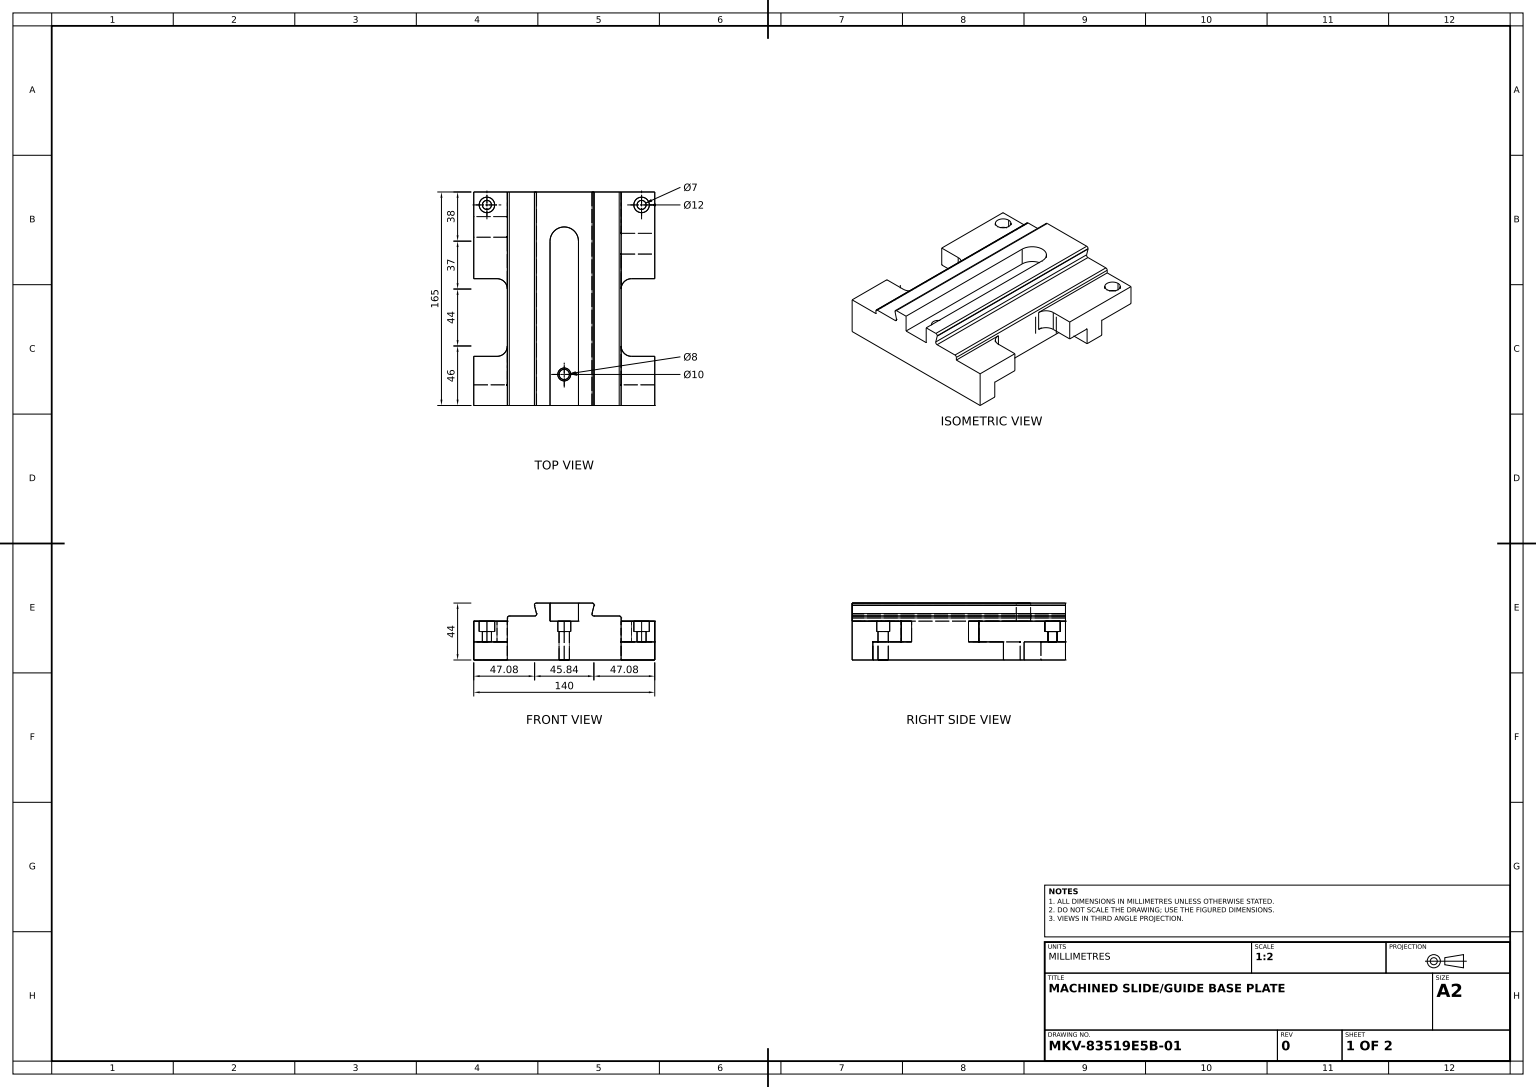
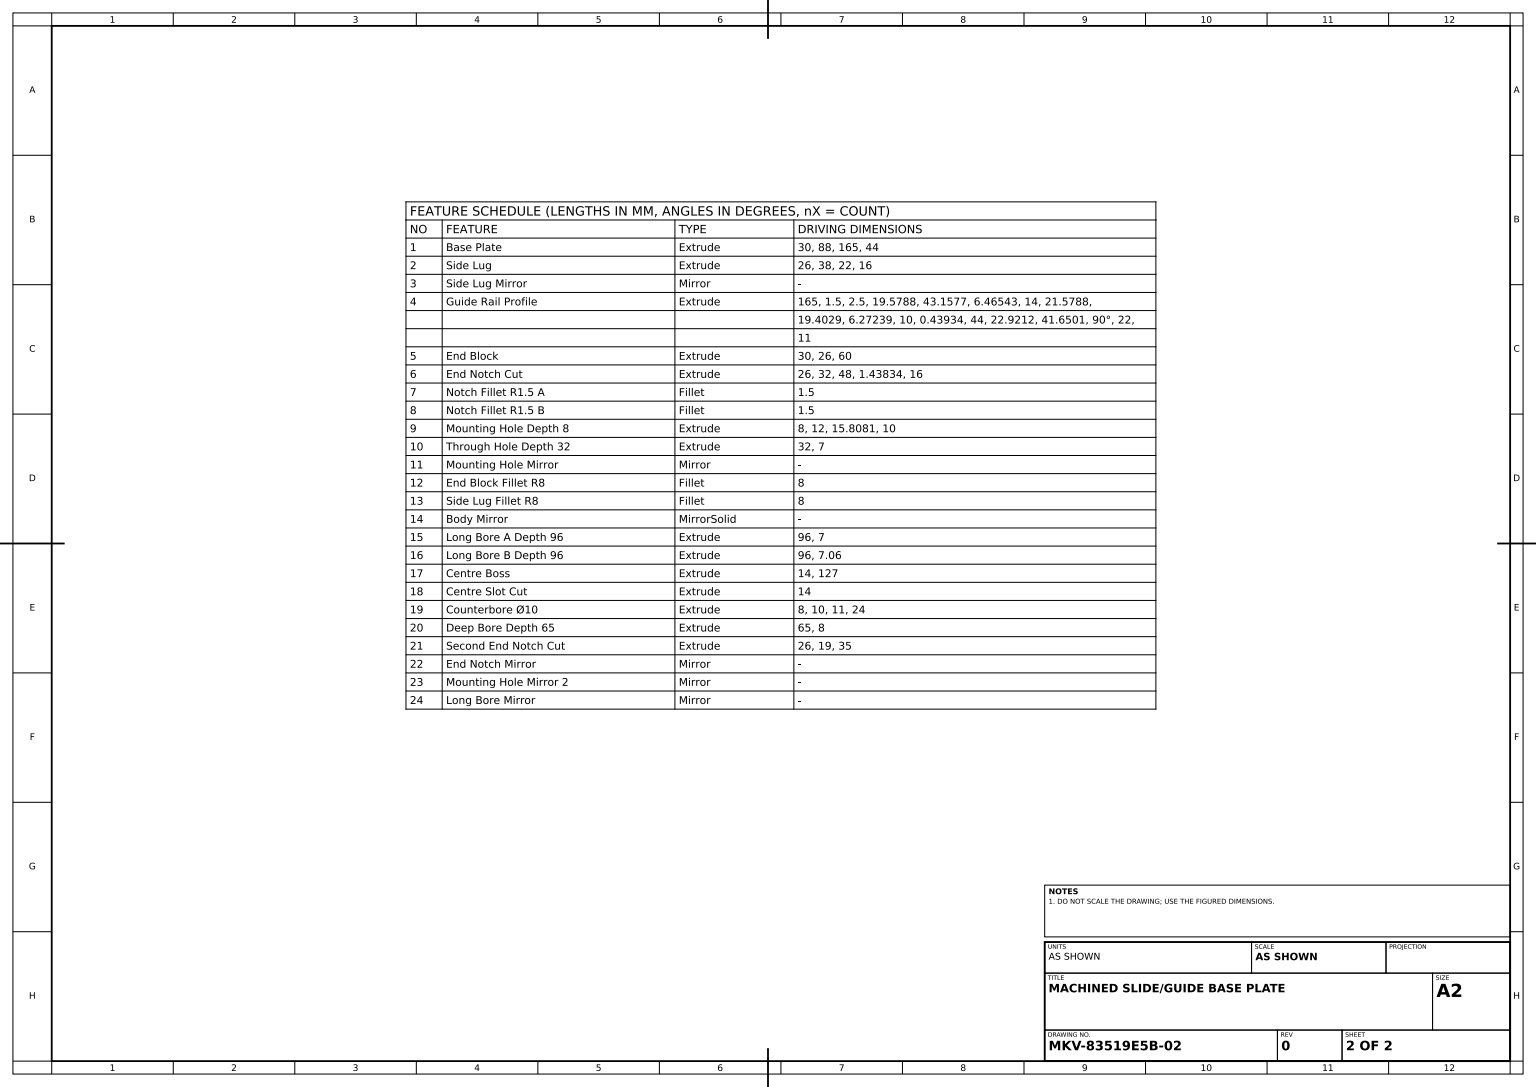
SolidWorks part; units mm, degrees
material "Plain Carbon Steel"
ref_plane "Front Plane" through (0, 0, 0) normal (0, 0, 1) x (1, 0, 0)
ref_plane "Top Plane" through (0, 0, 0) normal (0, 1, 0) x (1, 0, 0)
ref_plane "Right Plane" through (0, 0, 0) normal (1, 0, 0) x (0, 0, -1)
sketch "Base Plate Sketch" plane through (0, 0, 0) normal (0, 1, 0) x (1, 0, 0)
  line L2 (44, 0) -> (44, -82.5)
  line L3 (44, -82.5) -> (-44, -82.5)
  line L4 (-44, -82.5) -> (-44, 82.5)
  line L5 (-44, 82.5) -> (44, 82.5)
  line L6 (44, 82.5) -> (44, 0)
  dimension "D1" = 88
  dimension "D2" = 165
  dimension "D3" = 44
extrude "Base Plate" add sketch "Base Plate Sketch" against normal blind 30
sketch "Side Lug Sketch" plane through (44, 0, 0) normal (1, 0, 0) x (0, 0, -1)
  line L0 (-82.5, -30) -> (-82.5, 0)
  line L1 (-82.5, 0) -> (-44.5, 0)
  line L2 (-82.5, 0) -> (82.5, 0) construction
  line L3 (-44.5, 0) -> (-44.5, -16)
  line L4 (-82.5, -30) -> (-66.5, -30)
  line L5 (-82.5, -30) -> (82.5, -30) construction
  line L6 (-66.5, -30) -> (-66.5, -16)
  line L7 (-66.5, -16) -> (-44.5, -16)
  dimension "D1" = 38
  dimension "D2" = 30
  dimension "D3" = 22
  dimension "D4" = 16
extrude "Side Lug" add sketch "Side Lug Sketch" along normal blind 26
mirror "Side Lug Mirror" about plane through (0, 0, 0) normal (1, 0, 0) of "Side Lug"
sketch "Guide Rail Profile Sketch" plane through (0, 0, 82.5) normal (0, 0, 1) x (1, 0, 0)
  line L0 (0, 0) -> (44, 0)
  line L1 (-70, 0) -> (70, 0) construction
  line L2 (44, 0) -> (44, 2.5)
  line L4 (-21.5788, 14) -> (21.5788, 14)
  line L5 (42.5, 4) -> (22.9212, 4)
  line L7 (21.466, 5.8638) -> (23.034, 12.1362)
  line L8 (-44, 0) -> (-44, 2.5)
  line L9 (-42.5, 4) -> (-22.9212, 4)
  line L10 (-21.466, 5.8638) -> (-23.034, 12.1362)
  line L11 (0, 0) -> (-11, 0)
  line L12 (-11, 0) -> (-11, 14)
  line L13 (-11, 14) -> (11, 14)
  line L14 (11, 14) -> (11, 0)
  line L15 (11, 0) -> (-11, 0)
  line L16 (-44, 0) -> (-11, 0)
  arc A0 (44, 2.5) -> (42.5, 4) centre (42.5, 2.5) ccw
  arc A1 (22.9212, 4) -> (21.466, 5.8638) centre (22.9212, 5.5) cw
  arc A2 (21.5788, 14) -> (23.034, 12.1362) centre (21.5788, 12.5) cw
  arc A3 (-44, 2.5) -> (-42.5, 4) centre (-42.5, 2.5) cw
  arc A4 (-22.9212, 4) -> (-21.466, 5.8638) centre (-22.9212, 5.5) ccw
  arc A5 (-21.5788, 14) -> (-23.034, 12.1362) centre (-21.5788, 12.5) ccw
  point P7 (-43.5607, 3.5607)
  dimension "D1" = 1.5
  dimension "D2" = 1.5
  dimension "D4" = 1.5
  dimension "D7" = 1.5
  dimension "D12" = 21.5788
  dimension "D14" = 1.5
  dimension "D21" = 22.9212
  dimension "D23" = 22.9212
  dimension "D24" = 1.5
  dimension "D25" = 1.5
  dimension "D3" = 2.5
  dimension "D5" = 19.5788
  dimension "D6" = 43.1577
  dimension "D8" = 6.4654
  dimension "D9" = 19.5788
  dimension "D10" = 2.5
  dimension "D11" = 14
  dimension "D13" = 19.4029
  dimension "D15" = 19.4029
  dimension "D16" = 19.4029
  dimension "D17" = 6.2724
  dimension "D18" = 10
  dimension "D19" = 0.4393
  dimension "D20" = 44
  dimension "D22" = 41.6501
  dimension "D26" = 44
  dimension "D27" = 2.5
  dimension "D28" = 90
  dimension "D29" = 22
  dimension "D30" = 11
extrude "Guide Rail Profile" add sketch "Guide Rail Profile Sketch" against normal blind 165 contours A2 L4 L14 L12 L2 A0 L5 A1 L7 | L4 A5 L10 A4 L9 A3 L8 L12
sketch "End Block Sketch" plane through (0, 0, 0) normal (0, 1, 0) x (1, 0, 0)
  line L0 (-44, -44.5) -> (-44, -82.5) construction
  line L1 (-44, 15.5) -> (-70, 15.5)
  line L2 (-70, 15.5) -> (-70, 82.5)
  line L3 (-44, 15.5) -> (-44, 82.5)
  line L4 (-44, 82.5) -> (-70, 82.5)
  line L5 (-70, -44.5) -> (-44, -44.5) construction
  dimension "D1" = 26
  dimension "D2" = 60
extrude "End Block" add sketch "End Block Sketch" against normal blind 30
sketch "End Notch Sketch" plane through (-70, 0, 0) normal (-1, 0, 0) x (0, 0, 1)
  line L1 (-82.5, 0) -> (-15.5, 0) construction
  line L4 (-82.5, -30) -> (-50.5, -30)
  line L15 (-82.5, -30) -> (-15.5, -30) construction
  line L16 (-50.5, -30) -> (-50.5, -16)
  line L17 (-50.5, -16) -> (-34.5, -16)
  line L18 (-34.5, -16) -> (-34.5, -30)
  line L19 (-34.5, -30) -> (-15.5, -30)
  line L20 (-15.5, -30) -> (-15.5, 0)
  line L21 (-15.5, 0) -> (-82.5, 0)
  line L22 (-82.5, 0) -> (-82.5, -30)
  line L23 (-50.5, -16) -> (-83.9383, -16)
  line L24 (-34.5, -16) -> (-15.5, -16)
  line M8 (-82.5, -30) -> (-15.5, -30)
  line M9 (-15.5, -30) -> (-15.5, 0)
  dimension "D1" = 32
  dimension "D2" = 48
  dimension "D3" = 1.4383
  dimension "D4" = 16
extrude "End Notch Cut" cut sketch "End Notch Sketch" against normal blind 26 contours L24 L18 M8 M9 | L16 L23 L22 M8
fillet "Notch Fillet R1.5 A" radius 1.5 1 edges at (-57, -16, -50.5)
fillet "Notch Fillet R1.5 B" radius 1.5 1 edges at (-57, -16, -34.5)
sketch "Mounting Hole Sketch" plane through (0, 0, 0) normal (0, 1, 0) x (1, 0, 0)
  line L0 (-44, 15.5) -> (-44, 82.5) construction
  line L1 (-44, 82.5) -> (-70, 82.5) construction
  circle A1 centre (-59.8081, 72.5) radius 6
  dimension "D1" = 12
  dimension "D2" = 15.8081
  dimension "D3" = 10
extrude "Mounting Hole Depth 8" cut sketch "Mounting Hole Sketch" against normal blind 8
sketch "Through Hole Sketch" plane through (0, 0, 0) normal (0, 1, 0) x (1, 0, 0)
  circle A0 centre (-59.8081, 72.5) radius 3.5
  dimension "D1" = 7
extrude "Through Hole Depth 32" cut sketch "Through Hole Sketch" against normal blind 32
mirror "Mounting Hole Mirror" about plane through (0, 0, 0) normal (1, 0, 0) of "Mounting Hole Depth 8", "End Block"
fillet "End Block Fillet R8" radius 8 1 edges at (-44, -8, -15.5)
fillet "Side Lug Fillet R8" radius 8 1 edges at (-44, -8, 44.5)
mirror "Body Mirror" about plane through (0, 0, 0) normal (1, 0, 0) of bodies 114
sketch "Long Bore A Sketch" plane through (0, -8, 0) normal (0, 1, 0) x (1, 0, 0)
  circle A0 centre (-59.8081, 72.5) radius 3.5
  dimension "D1" = 7
extrude "Long Bore A Depth 96" cut sketch "Long Bore A Sketch" against normal blind 96
sketch "Long Bore B Sketch" plane through (0, -30, 0) normal (0, -1, 0) x (1, 0, 0)
  circle A0 centre (59.8081, -72.5) radius 3.53
  dimension "D1" = 7.06
extrude "Long Bore B Depth 96" cut sketch "Long Bore B Sketch" against normal blind 96
sketch "Centre Boss Sketch" plane through (0, 14, 0) normal (0, 1, 0) x (1, 0, 0)
  line L0 (-11, 82.5) -> (11, 82.5)
  line L1 (11, 82.5) -> (11, 44.5)
  line L2 (11, 82.5) -> (11, -82.5) construction
  line L3 (11, 44.5) -> (-11, 44.5)
  line L4 (-11, 82.5) -> (-11, -82.5) construction
  line L5 (-11, 44.5) -> (-11, 82.5)
  line L6 (-21.5788, -82.5) -> (-11, -82.5) construction
  dimension "D1" = 127
extrude "Centre Boss" add sketch "Centre Boss Sketch" against normal blind 14
sketch "Centre Slot Sketch" plane through (0, 14, 0) normal (0, 1, 0) x (1, 0, 0)
  line L0 (-11, 44.5) -> (11, 44.5) construction
  line L1 (-11, 44.5) -> (11, 44.5)
  arc A0 (11, 44.5) -> (-11, 44.5) centre (0, 44.5) ccw
extrude "Centre Slot Cut" cut sketch "Centre Slot Sketch" against normal blind 14
sketch "Counterbore Ø10 Sketch" plane through (0, 0, 0) normal (0, 1, 0) x (1, 0, 0)
  line L0 (11, 44.5) -> (11, -82.5) construction
  circle A0 centre (0, -58.5) radius 5
  dimension "D1" = 10
  dimension "D2" = 11
  dimension "D3" = 24
extrude "Counterbore Ø10" cut sketch "Counterbore Ø10 Sketch" against normal blind 8
sketch "Deep Bore Sketch" plane through (0, -8, 0) normal (0, 1, 0) x (1, 0, 0)
  circle A0 centre (0, -58.5) radius 4
  dimension "D1" = 8
extrude "Deep Bore Depth 65" cut sketch "Deep Bore Sketch" against normal blind 65
sketch "Second End Notch Sketch" plane through (-70, 0, 0) normal (-1, 0, 0) x (0, 0, 1)
  line L0 (-15.5, -30) -> (-47.5, -30)
  line L2 (-82.5, -30) -> (-15.5, -30) construction
  line L3 (-47.5, -30) -> (-47.5, -16)
  line L4 (-47.5, -16) -> (-63.5, -16)
  line L5 (-63.5, -16) -> (-63.5, -30)
  line L6 (-63.5, -30) -> (-82.5, -30)
  line L7 (-82.5, -30) -> (-82.5, 0)
  line L8 (-82.5, 0) -> (-15.5, 0)
  line L9 (-15.5, 0) -> (-15.5, -30)
  line L10 (-47.5, -16) -> (-15.5, -16)
  line L11 (-63.5, -16) -> (-82.5, -16)
  line M12 (-82.5, -30) -> (-15.5, -30)
  line M13 (-15.5, -30) -> (-15.5, 0)
  dimension "D1" = 19
  dimension "D2" = 35
extrude "Second End Notch Cut" cut sketch "Second End Notch Sketch" against normal blind 26 contours L10 L3 M12 M13 | L5 L11 L7 M12
mirror "End Notch Mirror" about plane through (0, 0, 0) normal (1, 0, 0) of "End Notch Cut", "End Block"
mirror "Mounting Hole Mirror 2" about plane through (0, 0, 0) normal (1, 0, 0) of "Mounting Hole Depth 8"
mirror "Long Bore Mirror" about plane through (0, 0, 0) normal (1, 0, 0) of "Long Bore A Depth 96"
